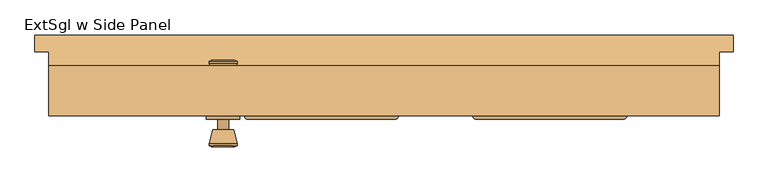
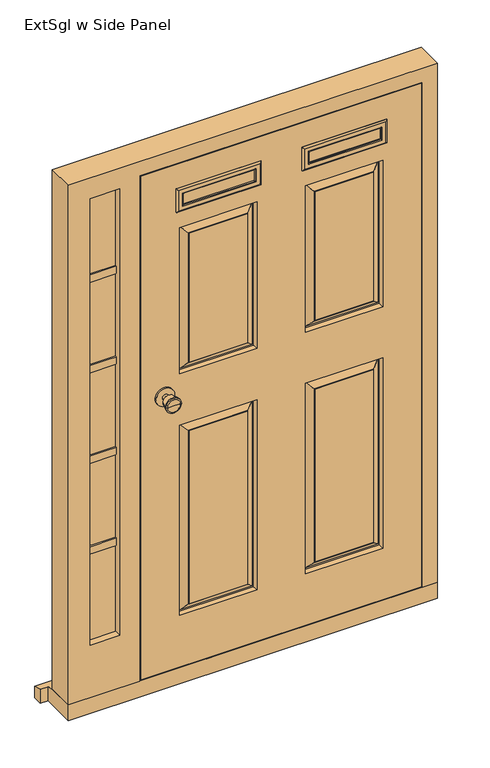
"""IFC4 building model written with IfcOpenShell, lengths in millimetres: door geometry, ExtSgl w Side Panel."""

from ifc_helpers import new_model, si_unit, point, frame, frame_2d, origin, place, context, project, spatial, polyline, circle_curve, ellipse_curve, trimmed, segment, composite_curve, outline, extrude, faceted_brep, source, transform, mapped, element, save
from ifc_brep_helpers import plane_surface, cylinder_surface, revolved_surface, advanced_brep


def extsgl_w_side_panel_d749231e(model_context):
    return source(origin(), model_context, "Body", "SolidModel", [
        advanced_brep(
        [(-518.7, -5.7, 1000.0), (-508.7, -5.7, 1000.0), (-528.7, -5.7, 1000.0), (-498.2241324, -54.7, 1000.0), (-518.7, -54.7, 1000.0), (-539.1758676, -54.7, 1000.0), (-493.7, -52.8721319, 1000.0), (-543.7, -52.8721319, 1000.0), (-493.7, -49.4084537, 1000.0), (-543.7, -49.4084537, 1000.0), (-500.063764, -24.7, 1000.0), (-537.336236, -24.7, 1000.0), (-508.7, -24.7, 1000.0), (-528.7, -24.7, 1000.0)],
        [
            (0, 1),
            (1, 2, circle_curve(frame((-518.7, -5.7, 1000.0), z_axis=(0.0, 1.0, 0.0), x_axis=(-1.0, 0.0, 0.0)), 10.0)),
            (2, 0),
            (2, 1, circle_curve(frame((-518.7, -5.7, 1000.0), z_axis=(0.0, 1.0, 0.0), x_axis=(-1.0, 0.0, 0.0)), 10.0)),
            (3, 4),
            (4, 5),
            (5, 3, circle_curve(frame((-518.7, -54.7, 1000.0), z_axis=(0.0, -1.0, 0.0), x_axis=(-1.0, 0.0, 0.0)), 20.4758676)),
            (3, 5, circle_curve(frame((-518.7, -54.7, 1000.0), z_axis=(0.0, -1.0, 0.0), x_axis=(-1.0, 0.0, 0.0)), 20.4758676)),
            (6, 3),
            (5, 7),
            (7, 6, circle_curve(frame((-518.7, -52.8721319, 1000.0), z_axis=(0.0, -1.0, 0.0), x_axis=(-1.0, 0.0, 0.0)), 25.0)),
            (6, 7, circle_curve(frame((-518.7, -52.8721319, 1000.0), z_axis=(0.0, -1.0, 0.0), x_axis=(-1.0, 0.0, 0.0)), 25.0)),
            (8, 6),
            (7, 9),
            (9, 8, circle_curve(frame((-518.7, -49.4084537, 1000.0), z_axis=(0.0, -1.0, 0.0), x_axis=(-1.0, 0.0, 0.0)), 25.0)),
            (8, 9, circle_curve(frame((-518.7, -49.4084537, 1000.0), z_axis=(0.0, -1.0, 0.0), x_axis=(-1.0, 0.0, 0.0)), 25.0)),
            (10, 8),
            (9, 11),
            (11, 10, circle_curve(frame((-518.7, -24.7, 1000.0), z_axis=(0.0, -1.0, 0.0), x_axis=(-1.0, 0.0, 0.0)), 18.636236)),
            (10, 11, circle_curve(frame((-518.7, -24.7, 1000.0), z_axis=(0.0, -1.0, 0.0), x_axis=(-1.0, 0.0, 0.0)), 18.636236)),
            (12, 10),
            (11, 13),
            (13, 12, circle_curve(frame((-518.7, -24.7, 1000.0), z_axis=(0.0, -1.0, 0.0), x_axis=(-1.0, 0.0, 0.0)), 10.0)),
            (12, 13, circle_curve(frame((-518.7, -24.7, 1000.0), z_axis=(0.0, -1.0, 0.0), x_axis=(-1.0, 0.0, 0.0)), 10.0)),
            (1, 12),
            (13, 2),
        ],
        [
            plane_surface(frame((-518.7, -5.7, 1000.0), z_axis=(0.0, 1.0, 0.0), x_axis=(-1.0, 0.0, 0.0))),
            plane_surface(frame((-518.7, -54.7, 1000.0), z_axis=(0.0, -1.0, 0.0), x_axis=(-1.0, 0.0, 0.0))),
            revolved_surface(polyline([(-539.1758676, -54.7, 1000.0), (-543.7, -52.8721319, 1000.0)]), (-518.7, -5.7, 1000.0), (0.0, 1.0, 0.0)),
            cylinder_surface(frame((-518.7, -5.7, 1000.0), z_axis=(0.0, 1.0, 0.0), x_axis=(-1.0, 0.0, 0.0)), 25.0),
            revolved_surface(polyline([(-543.7, -49.4084537, 1000.0), (-537.336236, -24.7, 1000.0)]), (-518.7, -5.7, 1000.0), (0.0, 1.0, 0.0)),
            plane_surface(frame((-518.7, -24.7, 1000.0), z_axis=(0.0, 1.0, 0.0), x_axis=(-1.0, 0.0, 0.0))),
            cylinder_surface(frame((-518.7, -5.7, 1000.0), z_axis=(0.0, 1.0, 0.0), x_axis=(-1.0, 0.0, 0.0)), 10.0),
        ],
        [
            (0, [[1, 2, 3]]),
            (0, [[-3, 4, -1]]),
            (1, [[5, 6, 7]]),
            (1, [[-6, -5, 8]]),
            (2, [[9, -7, 10, 11]]),
            (2, [[-10, -8, -9, 12]]),
            (3, [[13, -11, 14, 15]]),
            (3, [[-14, -12, -13, 16]]),
            (4, [[17, -15, 18, 19]]),
            (4, [[-18, -16, -17, 20]]),
            (5, [[21, -19, 22, 23]]),
            (5, [[-22, -20, -21, 24]]),
            (6, [[25, -23, 26, -2]]),
            (6, [[-26, -24, -25, -4]]),
        ],
    ),
        extrude(outline(composite_curve([segment(trimmed(circle_curve(frame_2d((1000.0, -518.7)), 30.0), [point((1000.0, -548.7))], [point((1000.0, -488.7))], False, "CARTESIAN"), True, "CONTINUOUS"), segment(trimmed(circle_curve(frame_2d((1000.0, -518.7)), 30.0), [point((1000.0, -488.7))], [point((1000.0, -548.7))], False, "CARTESIAN"), True, "CONTINUOUS")], self_intersect=False)), frame((0.0, -5.7, 0.0), z_axis=(0.0, 1.0, 0.0), x_axis=(0.0, 0.0, 1.0)), (0.0, 0.0, 1.0), 6.0),
        advanced_brep(
        [(-518.7, 50.3, 1000.0), (-528.7, 50.3, 1000.0), (-508.7, 50.3, 1000.0), (-498.2241324, 99.3, 1000.0), (-539.1758676, 99.3, 1000.0), (-518.7, 99.3, 1000.0), (-493.7, 97.4721319, 1000.0), (-543.7, 97.4721319, 1000.0), (-493.7, 94.0084537, 1000.0), (-543.7, 94.0084537, 1000.0), (-500.063764, 69.3, 1000.0), (-537.336236, 69.3, 1000.0), (-508.7, 69.3, 1000.0), (-528.7, 69.3, 1000.0)],
        [
            (0, 1),
            (1, 2, circle_curve(frame((-518.7, 50.3, 1000.0), z_axis=(0.0, -1.0, 0.0), x_axis=(-1.0, 0.0, 0.0)), 10.0)),
            (2, 0),
            (2, 1, circle_curve(frame((-518.7, 50.3, 1000.0), z_axis=(0.0, -1.0, 0.0), x_axis=(-1.0, 0.0, 0.0)), 10.0)),
            (3, 4, circle_curve(frame((-518.7, 99.3, 1000.0), z_axis=(0.0, 1.0, 0.0), x_axis=(-1.0, 0.0, 0.0)), 20.4758676)),
            (4, 5),
            (5, 3),
            (4, 3, circle_curve(frame((-518.7, 99.3, 1000.0), z_axis=(0.0, 1.0, 0.0), x_axis=(-1.0, 0.0, 0.0)), 20.4758676)),
            (6, 7, circle_curve(frame((-518.7, 97.4721319, 1000.0), z_axis=(0.0, 1.0, 0.0), x_axis=(-1.0, 0.0, 0.0)), 25.0)),
            (7, 4),
            (3, 6),
            (7, 6, circle_curve(frame((-518.7, 97.4721319, 1000.0), z_axis=(0.0, 1.0, 0.0), x_axis=(-1.0, 0.0, 0.0)), 25.0)),
            (8, 9, circle_curve(frame((-518.7, 94.0084537, 1000.0), z_axis=(0.0, 1.0, 0.0), x_axis=(-1.0, 0.0, 0.0)), 25.0)),
            (9, 7),
            (6, 8),
            (9, 8, circle_curve(frame((-518.7, 94.0084537, 1000.0), z_axis=(0.0, 1.0, 0.0), x_axis=(-1.0, 0.0, 0.0)), 25.0)),
            (10, 11, circle_curve(frame((-518.7, 69.3, 1000.0), z_axis=(0.0, 1.0, 0.0), x_axis=(-1.0, 0.0, 0.0)), 18.636236)),
            (11, 9),
            (8, 10),
            (11, 10, circle_curve(frame((-518.7, 69.3, 1000.0), z_axis=(0.0, 1.0, 0.0), x_axis=(-1.0, 0.0, 0.0)), 18.636236)),
            (12, 13, circle_curve(frame((-518.7, 69.3, 1000.0), z_axis=(0.0, 1.0, 0.0), x_axis=(-1.0, 0.0, 0.0)), 10.0)),
            (13, 11),
            (10, 12),
            (13, 12, circle_curve(frame((-518.7, 69.3, 1000.0), z_axis=(0.0, 1.0, 0.0), x_axis=(-1.0, 0.0, 0.0)), 10.0)),
            (1, 13),
            (12, 2),
        ],
        [
            plane_surface(frame((-518.7, 50.3, 1000.0), z_axis=(0.0, -1.0, 0.0), x_axis=(-1.0, 0.0, 0.0))),
            plane_surface(frame((-518.7, 99.3, 1000.0), z_axis=(0.0, 1.0, 0.0), x_axis=(-1.0, 0.0, 0.0))),
            revolved_surface(polyline([(-539.1758676, 99.3, 1000.0), (-543.7, 97.4721319, 1000.0)]), (-518.7, 50.3, 1000.0), (0.0, -1.0, 0.0)),
            cylinder_surface(frame((-518.7, 50.3, 1000.0), z_axis=(0.0, -1.0, 0.0), x_axis=(-1.0, 0.0, 0.0)), 25.0),
            revolved_surface(polyline([(-543.7, 94.0084537, 1000.0), (-537.336236, 69.3, 1000.0)]), (-518.7, 50.3, 1000.0), (0.0, -1.0, 0.0)),
            plane_surface(frame((-518.7, 69.3, 1000.0), z_axis=(0.0, -1.0, 0.0), x_axis=(-1.0, 0.0, 0.0))),
            cylinder_surface(frame((-518.7, 50.3, 1000.0), z_axis=(0.0, -1.0, 0.0), x_axis=(-1.0, 0.0, 0.0)), 10.0),
        ],
        [
            (0, [[1, 2, 3]]),
            (0, [[-3, 4, -1]]),
            (1, [[5, 6, 7]]),
            (1, [[8, -7, -6]]),
            (2, [[9, 10, -5, 11]]),
            (2, [[12, -11, -8, -10]]),
            (3, [[13, 14, -9, 15]]),
            (3, [[16, -15, -12, -14]]),
            (4, [[17, 18, -13, 19]]),
            (4, [[20, -19, -16, -18]]),
            (5, [[21, 22, -17, 23]]),
            (5, [[24, -23, -20, -22]]),
            (6, [[-2, 25, -21, 26]]),
            (6, [[-4, -26, -24, -25]]),
        ],
    ),
        extrude(outline(composite_curve([segment(trimmed(circle_curve(frame_2d((1000.0, -518.7)), 30.0), [point((1000.0, -548.7))], [point((1000.0, -488.7))], False, "CARTESIAN"), True, "CONTINUOUS"), segment(trimmed(circle_curve(frame_2d((1000.0, -518.7)), 30.0), [point((1000.0, -488.7))], [point((1000.0, -548.7))], False, "CARTESIAN"), True, "CONTINUOUS")], self_intersect=False)), frame((0.0, 44.3, 0.0), z_axis=(0.0, 1.0, 0.0), x_axis=(0.0, 0.0, 1.0)), (0.0, 0.0, 1.0), 6.0),
        faceted_brep([(294.3, 89.3, 54.5), (364.8, 89.3, 54.5), (364.8, 0.3, 54.5), (316.3, 0.3, 54.5), (316.3, 47.3, 54.5), (294.3, 47.3, 54.5), (294.3, 89.3, 1758.3), (-576.7, 89.3, 1758.3), (-576.7, 89.3, 54.5), (-829.0, 89.3, 54.5), (-829.0, 89.3, 1828.8), (364.8, 89.3, 1828.8), (-662.7, 89.3, 1758.3), (-758.5, 89.3, 1758.3), (-758.5, 89.3, 233.5), (-662.7, 89.3, 233.5), (364.8, 0.3, 1828.8), (-829.0, 0.3, 1828.8), (-829.0, 0.3, 54.5), (-598.7, 0.3, 54.5), (-598.7, 0.3, 1780.3), (316.3, 0.3, 1780.3), (-662.7, 0.3, 233.5), (-758.5, 0.3, 233.5), (-758.5, 0.3, 1758.3), (-662.7, 0.3, 1758.3), (316.3, 47.3, 1780.3), (-598.7, 47.3, 1780.3), (-598.7, 47.3, 54.5), (-576.7, 47.3, 54.5), (-576.7, 47.3, 1758.3), (294.3, 47.3, 1758.3), (-640.7, 47.3, 1780.3), (-780.5, 47.3, 1780.3), (-780.5, 47.3, 218.5), (-640.7, 47.3, 218.5), (-758.5, 47.3, 1758.3), (-662.7, 47.3, 1758.3), (-662.7, 47.3, 233.5), (-758.5, 47.3, 233.5), (-662.7, 23.3, 233.5), (-758.5, 23.3, 233.5), (-758.5, 23.3, 1758.3), (-662.7, 23.3, 1758.3), (-780.5, 23.3, 1780.3), (-780.5, 23.3, 218.5), (-640.7, 23.3, 218.5), (-640.7, 23.3, 1780.3)], [[[0, 1, 2, 3, 4, 5]], [[1, 0, 6, 7, 8, 9, 10, 11], [12, 13, 14, 15]], [[2, 1, 11, 16]], [[3, 2, 16, 17, 18, 19, 20, 21], [22, 23, 24, 25]], [[4, 3, 21, 26]], [[5, 4, 26, 27, 28, 29, 30, 31]], [[32, 33, 34, 35], [36, 37, 38, 39]], [[0, 5, 31, 6]], [[29, 8, 7, 30]], [[18, 9, 8, 29, 28, 19]], [[10, 9, 18, 17]], [[13, 36, 39, 14]], [[39, 38, 15, 14]], [[37, 12, 15, 38]], [[23, 22, 40, 41]], [[24, 23, 41, 42]], [[22, 25, 43, 40]], [[19, 28, 27, 20]], [[44, 45, 34, 33]], [[45, 46, 35, 34]], [[46, 47, 32, 35]], [[46, 45, 44, 47], [41, 40, 43, 42]], [[11, 10, 17, 16]], [[26, 21, 20, 27]], [[33, 32, 47, 44]], [[6, 31, 30, 7]], [[36, 13, 12, 37]], [[25, 24, 42, 43]]]),
        faceted_brep([(313.3, 0.3, 58.5), (313.3, 0.3, 1777.3), (-593.7, 0.3, 1777.3), (-593.7, 0.3, 58.5), (-61.7, 0.3, 1683.5), (188.3, 0.3, 1683.5), (188.3, 0.3, 1627.3), (-61.7, 0.3, 1627.3), (-468.7, 0.3, 1683.5), (-218.7, 0.3, 1683.5), (-218.7, 0.3, 1627.3), (-468.7, 0.3, 1627.3), (-218.7, 0.3, 883.5), (-218.7, 0.3, 233.5), (-468.7, 0.3, 233.5), (-468.7, 0.3, 883.5), (188.3, 0.3, 883.5), (188.3, 0.3, 233.5), (-61.7, 0.3, 233.5), (-61.7, 0.3, 883.5), (-218.7, 0.3, 1558.5), (-218.7, 0.3, 1058.5), (-468.7, 0.3, 1058.5), (-468.7, 0.3, 1558.5), (188.3, 0.3, 1558.5), (188.3, 0.3, 1058.5), (-61.7, 0.3, 1058.5), (-61.7, 0.3, 1558.5), (-248.7, 0.3, 263.5), (-248.7, 0.3, 853.5), (-438.7, 0.3, 853.5), (-438.7, 0.3, 263.5), (158.3, 0.3, 263.5), (158.3, 0.3, 853.5), (-31.7, 0.3, 853.5), (-31.7, 0.3, 263.5), (-248.7, 0.3, 1088.5), (-248.7, 0.3, 1528.5), (-438.7, 0.3, 1528.5), (-438.7, 0.3, 1088.5), (158.3, 0.3, 1088.5), (158.3, 0.3, 1528.5), (-31.7, 0.3, 1528.5), (-31.7, 0.3, 1088.5), (313.3, 44.3, 58.5), (-593.7, 44.3, 58.5), (-593.7, 44.3, 1777.3), (313.3, 44.3, 1777.3), (-61.7, 44.3, 1683.5), (-61.7, 44.3, 1627.3), (188.3, 44.3, 1627.3), (188.3, 44.3, 1683.5), (-468.7, 44.3, 1683.5), (-468.7, 44.3, 1627.3), (-218.7, 44.3, 1627.3), (-218.7, 44.3, 1683.5), (-61.7, 44.3, 883.5), (-61.7, 44.3, 233.5), (188.3, 44.3, 233.5), (188.3, 44.3, 883.5), (-468.7, 44.3, 883.5), (-468.7, 44.3, 233.5), (-218.7, 44.3, 233.5), (-218.7, 44.3, 883.5), (-61.7, 44.3, 1558.5), (-61.7, 44.3, 1058.5), (188.3, 44.3, 1058.5), (188.3, 44.3, 1558.5), (-468.7, 44.3, 1558.5), (-468.7, 44.3, 1058.5), (-218.7, 44.3, 1058.5), (-218.7, 44.3, 1558.5), (-31.7, 44.3, 263.5), (-31.7, 44.3, 853.5), (158.3, 44.3, 853.5), (158.3, 44.3, 263.5), (-438.7, 44.3, 263.5), (-438.7, 44.3, 853.5), (-248.7, 44.3, 853.5), (-248.7, 44.3, 263.5), (-31.7, 44.3, 1088.5), (-31.7, 44.3, 1528.5), (158.3, 44.3, 1528.5), (158.3, 44.3, 1088.5), (-438.7, 44.3, 1088.5), (-438.7, 44.3, 1528.5), (-248.7, 44.3, 1528.5), (-248.7, 44.3, 1088.5), (-58.7, 29.3, 880.5), (-58.7, 29.3, 236.5), (-33.7, 43.3, 855.5), (-33.7, 43.3, 261.5), (-53.7, 29.3, 241.5), (-53.7, 29.3, 875.5), (-31.7, 43.3, 263.5), (-31.7, 43.3, 853.5), (185.3, 29.3, 236.5), (160.3, 43.3, 261.5), (180.3, 29.3, 241.5), (158.3, 43.3, 263.5), (185.3, 29.3, 880.5), (160.3, 43.3, 855.5), (180.3, 29.3, 875.5), (158.3, 43.3, 853.5), (-465.7, 29.3, 880.5), (-465.7, 29.3, 236.5), (-440.7, 43.3, 855.5), (-440.7, 43.3, 261.5), (-460.7, 29.3, 241.5), (-460.7, 29.3, 875.5), (-438.7, 43.3, 263.5), (-438.7, 43.3, 853.5), (-221.7, 29.3, 236.5), (-246.7, 43.3, 261.5), (-226.7, 29.3, 241.5), (-248.7, 43.3, 263.5), (-221.7, 29.3, 880.5), (-246.7, 43.3, 855.5), (-226.7, 29.3, 875.5), (-248.7, 43.3, 853.5), (-248.7, 1.3, 263.5), (-248.7, 1.3, 853.5), (-226.7, 15.3, 241.5), (-226.7, 15.3, 875.5), (-246.7, 1.3, 855.5), (-246.7, 1.3, 261.5), (-221.7, 15.3, 880.5), (-221.7, 15.3, 236.5), (-438.7, 1.3, 853.5), (-460.7, 15.3, 875.5), (-440.7, 1.3, 855.5), (-465.7, 15.3, 880.5), (-438.7, 1.3, 263.5), (-460.7, 15.3, 241.5), (-440.7, 1.3, 261.5), (-465.7, 15.3, 236.5), (185.3, 15.3, 880.5), (185.3, 15.3, 236.5), (160.3, 1.3, 855.5), (160.3, 1.3, 261.5), (180.3, 15.3, 241.5), (180.3, 15.3, 875.5), (158.3, 1.3, 263.5), (158.3, 1.3, 853.5), (-58.7, 15.3, 236.5), (-33.7, 1.3, 261.5), (-53.7, 15.3, 241.5), (-31.7, 1.3, 263.5), (-58.7, 15.3, 880.5), (-33.7, 1.3, 855.5), (-53.7, 15.3, 875.5), (-31.7, 1.3, 853.5), (-31.7, 43.3, 1088.5), (-31.7, 43.3, 1528.5), (-53.7, 29.3, 1066.5), (-53.7, 29.3, 1550.5), (-33.7, 43.3, 1530.5), (-33.7, 43.3, 1086.5), (-58.7, 29.3, 1555.5), (-58.7, 29.3, 1061.5), (158.3, 43.3, 1528.5), (180.3, 29.3, 1550.5), (160.3, 43.3, 1530.5), (185.3, 29.3, 1555.5), (158.3, 43.3, 1088.5), (180.3, 29.3, 1066.5), (160.3, 43.3, 1086.5), (185.3, 29.3, 1061.5), (-438.7, 43.3, 1088.5), (-438.7, 43.3, 1528.5), (-460.7, 29.3, 1066.5), (-460.7, 29.3, 1550.5), (-440.7, 43.3, 1530.5), (-440.7, 43.3, 1086.5), (-465.7, 29.3, 1555.5), (-465.7, 29.3, 1061.5), (-248.7, 43.3, 1528.5), (-226.7, 29.3, 1550.5), (-246.7, 43.3, 1530.5), (-221.7, 29.3, 1555.5), (-248.7, 43.3, 1088.5), (-226.7, 29.3, 1066.5), (-246.7, 43.3, 1086.5), (-221.7, 29.3, 1061.5), (-248.7, 1.3, 1088.5), (-248.7, 1.3, 1528.5), (-226.7, 15.3, 1066.5), (-226.7, 15.3, 1550.5), (-246.7, 1.3, 1530.5), (-246.7, 1.3, 1086.5), (-221.7, 15.3, 1555.5), (-221.7, 15.3, 1061.5), (-438.7, 1.3, 1528.5), (-460.7, 15.3, 1550.5), (-440.7, 1.3, 1530.5), (-465.7, 15.3, 1555.5), (-438.7, 1.3, 1088.5), (-460.7, 15.3, 1066.5), (-440.7, 1.3, 1086.5), (-465.7, 15.3, 1061.5), (185.3, 15.3, 1555.5), (185.3, 15.3, 1061.5), (160.3, 1.3, 1530.5), (160.3, 1.3, 1086.5), (180.3, 15.3, 1066.5), (180.3, 15.3, 1550.5), (158.3, 1.3, 1088.5), (158.3, 1.3, 1528.5), (-58.7, 15.3, 1061.5), (-33.7, 1.3, 1086.5), (-53.7, 15.3, 1066.5), (-31.7, 1.3, 1088.5), (-58.7, 15.3, 1555.5), (-33.7, 1.3, 1530.5), (-53.7, 15.3, 1550.5), (-31.7, 1.3, 1528.5)], [[[0, 1, 2, 3], [4, 5, 6, 7], [8, 9, 10, 11], [12, 13, 14, 15], [16, 17, 18, 19], [20, 21, 22, 23], [24, 25, 26, 27]], [[28, 29, 30, 31]], [[32, 33, 34, 35]], [[36, 37, 38, 39]], [[40, 41, 42, 43]], [[44, 45, 46, 47], [48, 49, 50, 51], [52, 53, 54, 55], [56, 57, 58, 59], [60, 61, 62, 63], [64, 65, 66, 67], [68, 69, 70, 71]], [[72, 73, 74, 75]], [[76, 77, 78, 79]], [[80, 81, 82, 83]], [[84, 85, 86, 87]], [[1, 0, 44, 47]], [[2, 1, 47, 46]], [[3, 2, 46, 45]], [[0, 3, 45, 44]], [[4, 7, 49, 48]], [[7, 6, 50, 49]], [[6, 5, 51, 50]], [[5, 4, 48, 51]], [[8, 11, 53, 52]], [[11, 10, 54, 53]], [[10, 9, 55, 54]], [[9, 8, 52, 55]], [[88, 89, 57, 56]], [[90, 91, 92, 93]], [[72, 94, 95, 73]], [[57, 89, 96, 58]], [[92, 91, 97, 98]], [[94, 72, 75, 99]], [[58, 96, 100, 59]], [[98, 97, 101, 102]], [[99, 75, 74, 103]], [[88, 56, 59, 100]], [[89, 88, 100, 96], [93, 92, 98, 102]], [[90, 93, 102, 101]], [[91, 90, 101, 97], [95, 94, 99, 103]], [[73, 95, 103, 74]], [[104, 105, 61, 60]], [[106, 107, 108, 109]], [[76, 110, 111, 77]], [[61, 105, 112, 62]], [[108, 107, 113, 114]], [[110, 76, 79, 115]], [[62, 112, 116, 63]], [[114, 113, 117, 118]], [[115, 79, 78, 119]], [[104, 60, 63, 116]], [[105, 104, 116, 112], [109, 108, 114, 118]], [[106, 109, 118, 117]], [[107, 106, 117, 113], [111, 110, 115, 119]], [[77, 111, 119, 78]], [[120, 121, 29, 28]], [[122, 123, 124, 125]], [[12, 126, 127, 13]], [[29, 121, 128, 30]], [[124, 123, 129, 130]], [[126, 12, 15, 131]], [[30, 128, 132, 31]], [[130, 129, 133, 134]], [[131, 15, 14, 135]], [[120, 28, 31, 132]], [[125, 124, 130, 134], [121, 120, 132, 128]], [[122, 125, 134, 133]], [[127, 126, 131, 135], [123, 122, 133, 129]], [[13, 127, 135, 14]], [[136, 137, 17, 16]], [[138, 139, 140, 141]], [[32, 142, 143, 33]], [[17, 137, 144, 18]], [[140, 139, 145, 146]], [[142, 32, 35, 147]], [[18, 144, 148, 19]], [[146, 145, 149, 150]], [[147, 35, 34, 151]], [[136, 16, 19, 148]], [[137, 136, 148, 144], [141, 140, 146, 150]], [[138, 141, 150, 149]], [[139, 138, 149, 145], [143, 142, 147, 151]], [[33, 143, 151, 34]], [[152, 153, 81, 80]], [[154, 155, 156, 157]], [[64, 158, 159, 65]], [[81, 153, 160, 82]], [[156, 155, 161, 162]], [[158, 64, 67, 163]], [[82, 160, 164, 83]], [[162, 161, 165, 166]], [[163, 67, 66, 167]], [[152, 80, 83, 164]], [[157, 156, 162, 166], [153, 152, 164, 160]], [[154, 157, 166, 165]], [[159, 158, 163, 167], [155, 154, 165, 161]], [[65, 159, 167, 66]], [[168, 169, 85, 84]], [[170, 171, 172, 173]], [[68, 174, 175, 69]], [[85, 169, 176, 86]], [[172, 171, 177, 178]], [[174, 68, 71, 179]], [[86, 176, 180, 87]], [[178, 177, 181, 182]], [[179, 71, 70, 183]], [[168, 84, 87, 180]], [[173, 172, 178, 182], [169, 168, 180, 176]], [[170, 173, 182, 181]], [[175, 174, 179, 183], [171, 170, 181, 177]], [[69, 175, 183, 70]], [[184, 185, 37, 36]], [[186, 187, 188, 189]], [[20, 190, 191, 21]], [[37, 185, 192, 38]], [[188, 187, 193, 194]], [[190, 20, 23, 195]], [[38, 192, 196, 39]], [[194, 193, 197, 198]], [[195, 23, 22, 199]], [[184, 36, 39, 196]], [[189, 188, 194, 198], [185, 184, 196, 192]], [[186, 189, 198, 197]], [[191, 190, 195, 199], [187, 186, 197, 193]], [[21, 191, 199, 22]], [[200, 201, 25, 24]], [[202, 203, 204, 205]], [[40, 206, 207, 41]], [[25, 201, 208, 26]], [[204, 203, 209, 210]], [[206, 40, 43, 211]], [[26, 208, 212, 27]], [[210, 209, 213, 214]], [[211, 43, 42, 215]], [[200, 24, 27, 212]], [[201, 200, 212, 208], [205, 204, 210, 214]], [[202, 205, 214, 213]], [[203, 202, 213, 209], [207, 206, 211, 215]], [[41, 207, 215, 42]]]),
        faceted_brep([(389.8, 144.3, 0.0), (389.8, 144.3, 38.5947221), (389.8, 114.3, 47.2703282), (389.8, 114.3, 0.0), (-854.0, 144.3, 38.5947221), (-854.0, 144.3, 0.0), (-854.0, 114.3, 0.0), (-854.0, 114.3, 47.2703282), (364.8, 114.3, 0.0), (364.8, 0.3, 0.0), (-829.0, 0.3, 0.0), (-829.0, 114.3, 0.0), (-829.0, 114.3, 47.2703282), (-829.0, 89.3, 54.5), (364.8, 89.3, 54.5), (364.8, 114.3, 47.2703282), (-829.0, 0.3, 54.5), (364.8, 0.3, 54.5)], [[[0, 1, 2, 3]], [[4, 5, 6, 7]], [[5, 0, 3, 8, 9, 10, 11, 6]], [[1, 0, 5, 4]], [[1, 4, 7, 12, 13, 14, 15, 2]], [[13, 16, 17, 14]], [[16, 10, 9, 17]], [[12, 11, 10, 16, 13]], [[11, 12, 7, 6]], [[8, 15, 14, 17, 9]], [[15, 8, 3, 2]]]),
        extrude(outline(polyline([(188.3, 10.3), (-61.7, 10.3), (-61.7, 34.3), (188.3, 34.3), (188.3, 10.3)])), frame((0.0, 0.0, 1627.3), z_axis=(0.0, 0.0, 1.0), x_axis=(1.0, 0.0, 0.0)), (0.0, 0.0, 1.0), 56.2),
        extrude(outline(polyline([(-218.7, 10.3), (-468.7, 10.3), (-468.7, 34.3), (-218.7, 34.3), (-218.7, 10.3)])), frame((0.0, 0.0, 1627.3), z_axis=(0.0, 0.0, 1.0), x_axis=(1.0, 0.0, 0.0)), (0.0, 0.0, 1.0), 56.2),
        advanced_brep(
        [(-53.7, 48.3, 1675.5), (-53.7, 44.3, 1675.5), (-53.7, 44.3, 1635.3), (-53.7, 48.3, 1635.3), (-55.7, 50.3, 1677.5), (-55.7, 50.3, 1633.3), (-73.7, 45.3, 1695.5), (-68.7, 50.3, 1690.5), (-68.7, 50.3, 1620.3), (-73.7, 45.3, 1615.3), (-73.7, 34.3, 1695.5), (-73.7, 34.3, 1615.3), (-61.7, 44.3, 1683.5), (-61.7, 34.3, 1683.5), (-61.7, 34.3, 1627.3), (-61.7, 44.3, 1627.3), (180.3, 44.3, 1635.3), (180.3, 48.3, 1635.3), (182.3, 50.3, 1633.3), (195.3, 50.3, 1620.3), (200.3, 45.3, 1615.3), (200.3, 34.3, 1615.3), (188.3, 34.3, 1627.3), (188.3, 44.3, 1627.3), (180.3, 44.3, 1675.5), (180.3, 48.3, 1675.5), (182.3, 50.3, 1677.5), (195.3, 50.3, 1690.5), (200.3, 45.3, 1695.5), (200.3, 34.3, 1695.5), (188.3, 34.3, 1683.5), (188.3, 44.3, 1683.5)],
        [
            (0, 1),
            (1, 2),
            (2, 3),
            (3, 0),
            (4, 0, ellipse_curve(frame((-55.7, 48.3, 1677.5), z_axis=(-0.7071067811865475, 0.0, -0.7071067811865475), x_axis=(-0.7071067811865474, 0.0, 0.7071067811865476)), 2.8284271, 2.0)),
            (3, 5, ellipse_curve(frame((-55.7, 48.3, 1633.3), z_axis=(-0.7071067811865475, 0.0, 0.7071067811865475), x_axis=(0.7071067811865474, 0.0, 0.7071067811865476)), 2.8284271, 2.0)),
            (5, 4),
            (6, 7, ellipse_curve(frame((-68.7, 45.3, 1690.5), z_axis=(-0.7071067811865475, 0.0, -0.7071067811865475), x_axis=(-0.7071067811865474, 0.0, 0.7071067811865476)), 7.0710678, 5.0)),
            (7, 8),
            (8, 9, ellipse_curve(frame((-68.7, 45.3, 1620.3), z_axis=(-0.7071067811865475, 0.0, 0.7071067811865475), x_axis=(0.7071067811865474, 0.0, 0.7071067811865476)), 7.0710678, 5.0)),
            (9, 6),
            (10, 6),
            (9, 11),
            (11, 10),
            (12, 13),
            (13, 14),
            (14, 15),
            (15, 12),
            (2, 16),
            (16, 17),
            (17, 3),
            (17, 18, ellipse_curve(frame((182.3, 48.3, 1633.3), z_axis=(-0.7071067811865475, 0.0, -0.7071067811865475), x_axis=(-0.7071067811865476, 0.0, 0.7071067811865474)), 2.8284271, 2.0)),
            (18, 5),
            (8, 19),
            (19, 20, ellipse_curve(frame((195.3, 45.3, 1620.3), z_axis=(-0.7071067811865475, 0.0, -0.7071067811865475), x_axis=(-0.7071067811865476, 0.0, 0.7071067811865474)), 7.0710678, 5.0)),
            (20, 9),
            (20, 21),
            (21, 11),
            (14, 22),
            (22, 23),
            (23, 15),
            (16, 24),
            (24, 25),
            (25, 17),
            (25, 26, ellipse_curve(frame((182.3, 48.3, 1677.5), z_axis=(0.7071067811865475, 0.0, -0.7071067811865475), x_axis=(-0.7071067811865474, 0.0, -0.7071067811865476)), 2.8284271, 2.0)),
            (26, 18),
            (19, 27),
            (27, 28, ellipse_curve(frame((195.3, 45.3, 1690.5), z_axis=(0.7071067811865475, 0.0, -0.7071067811865475), x_axis=(-0.7071067811865474, 0.0, -0.7071067811865476)), 7.0710678, 5.0)),
            (28, 20),
            (28, 29),
            (29, 21),
            (22, 30),
            (30, 31),
            (31, 23),
            (24, 1),
            (0, 25),
            (4, 26),
            (7, 27),
            (6, 28),
            (10, 29),
            (13, 30),
            (12, 31),
        ],
        [
            plane_surface(frame((-53.7, 44.3, 1675.5), z_axis=(1.0, 0.0, 0.0), x_axis=(0.0, 0.0, -1.0))),
            cylinder_surface(frame((-55.7, 48.3, 1683.5), z_axis=(0.0, 0.0, 1.0), x_axis=(1.0, 0.0, 0.0)), 2.0),
            cylinder_surface(frame((-68.7, 45.3, 1683.5), z_axis=(0.0, 0.0, 1.0), x_axis=(1.0, 0.0, 0.0)), 5.0),
            plane_surface(frame((-73.7, 45.3, 1695.5), z_axis=(-1.0, 0.0, 0.0), x_axis=(0.0, 0.0, -1.0))),
            plane_surface(frame((-61.7, 34.3, 1683.5), z_axis=(1.0, 0.0, 0.0), x_axis=(0.0, 0.0, -1.0))),
            plane_surface(frame((-53.7, 44.3, 1635.3), z_axis=(0.0, 0.0, 1.0), x_axis=(1.0, 0.0, 0.0))),
            cylinder_surface(frame((-61.7, 48.3, 1633.3), z_axis=(-1.0, 0.0, 0.0), x_axis=(0.0, 0.0, 1.0)), 2.0),
            cylinder_surface(frame((-61.7, 45.3, 1620.3), z_axis=(-1.0, 0.0, 0.0), x_axis=(0.0, 0.0, 1.0)), 5.0),
            plane_surface(frame((-73.7, 45.3, 1615.3), z_axis=(0.0, 0.0, -1.0), x_axis=(1.0, 0.0, 0.0))),
            plane_surface(frame((-61.7, 34.3, 1627.3), z_axis=(0.0, 0.0, 1.0), x_axis=(1.0, 0.0, 0.0))),
            plane_surface(frame((180.3, 44.3, 1635.3), z_axis=(-1.0, 0.0, 0.0), x_axis=(0.0, 0.0, 1.0))),
            cylinder_surface(frame((182.3, 48.3, 1627.3), z_axis=(0.0, 0.0, -1.0), x_axis=(-1.0, 0.0, 0.0)), 2.0),
            cylinder_surface(frame((195.3, 45.3, 1627.3), z_axis=(0.0, 0.0, -1.0), x_axis=(-1.0, 0.0, 0.0)), 5.0),
            plane_surface(frame((200.3, 45.3, 1615.3), z_axis=(1.0, 0.0, 0.0), x_axis=(0.0, 0.0, 1.0))),
            plane_surface(frame((188.3, 34.3, 1627.3), z_axis=(-1.0, 0.0, 0.0), x_axis=(0.0, 0.0, 1.0))),
            plane_surface(frame((180.3, 44.3, 1675.5), z_axis=(0.0, 0.0, -1.0), x_axis=(-1.0, 0.0, 0.0))),
            cylinder_surface(frame((188.3, 48.3, 1677.5), z_axis=(1.0, 0.0, 0.0), x_axis=(0.0, 0.0, -1.0)), 2.0),
            plane_surface(frame((182.3, 50.3, 1677.5), z_axis=(0.0, 1.0, 0.0), x_axis=(-1.0, 0.0, 0.0))),
            cylinder_surface(frame((188.3, 45.3, 1690.5), z_axis=(1.0, 0.0, 0.0), x_axis=(0.0, 0.0, -1.0)), 5.0),
            plane_surface(frame((200.3, 45.3, 1695.5), z_axis=(0.0, 0.0, 1.0), x_axis=(-1.0, 0.0, 0.0))),
            plane_surface(frame((200.3, 34.3, 1695.5), z_axis=(0.0, -1.0, 0.0), x_axis=(-1.0, 0.0, 0.0))),
            plane_surface(frame((188.3, 34.3, 1683.5), z_axis=(0.0, 0.0, -1.0), x_axis=(-1.0, 0.0, 0.0))),
            plane_surface(frame((188.3, 44.3, 1683.5), z_axis=(0.0, -1.0, 0.0), x_axis=(-1.0, 0.0, 0.0))),
        ],
        [
            (0, [[1, 2, 3, 4]]),
            (1, [[5, -4, 6, 7]]),
            (2, [[8, 9, 10, 11]]),
            (3, [[12, -11, 13, 14]]),
            (4, [[15, 16, 17, 18]]),
            (5, [[-3, 19, 20, 21]]),
            (6, [[-6, -21, 22, 23]]),
            (7, [[-10, 24, 25, 26]]),
            (8, [[-13, -26, 27, 28]]),
            (9, [[-17, 29, 30, 31]]),
            (10, [[-20, 32, 33, 34]]),
            (11, [[-22, -34, 35, 36]]),
            (12, [[-25, 37, 38, 39]]),
            (13, [[-27, -39, 40, 41]]),
            (14, [[-30, 42, 43, 44]]),
            (15, [[-33, 45, -1, 46]]),
            (16, [[-35, -46, -5, 47]]),
            (17, [[48, -37, -24, -9], [-23, -36, -47, -7]]),
            (18, [[-38, -48, -8, 49]]),
            (19, [[-40, -49, -12, 50]]),
            (20, [[-28, -41, -50, -14], [51, -42, -29, -16]]),
            (21, [[-43, -51, -15, 52]]),
            (22, [[-31, -44, -52, -18], [-45, -32, -19, -2]]),
        ],
    ),
        advanced_brep(
        [(-460.7, 48.3, 1675.5), (-460.7, 44.3, 1675.5), (-460.7, 44.3, 1635.3), (-460.7, 48.3, 1635.3), (-462.7, 50.3, 1677.5), (-462.7, 50.3, 1633.3), (-480.7, 45.3, 1695.5), (-475.7, 50.3, 1690.5), (-475.7, 50.3, 1620.3), (-480.7, 45.3, 1615.3), (-480.7, 34.3, 1695.5), (-480.7, 34.3, 1615.3), (-468.7, 44.3, 1683.5), (-468.7, 34.3, 1683.5), (-468.7, 34.3, 1627.3), (-468.7, 44.3, 1627.3), (-226.7, 44.3, 1635.3), (-226.7, 48.3, 1635.3), (-224.7, 50.3, 1633.3), (-211.7, 50.3, 1620.3), (-206.7, 45.3, 1615.3), (-206.7, 34.3, 1615.3), (-218.7, 34.3, 1627.3), (-218.7, 44.3, 1627.3), (-226.7, 44.3, 1675.5), (-226.7, 48.3, 1675.5), (-224.7, 50.3, 1677.5), (-211.7, 50.3, 1690.5), (-206.7, 45.3, 1695.5), (-206.7, 34.3, 1695.5), (-218.7, 34.3, 1683.5), (-218.7, 44.3, 1683.5)],
        [
            (0, 1),
            (1, 2),
            (2, 3),
            (3, 0),
            (4, 0, ellipse_curve(frame((-462.7, 48.3, 1677.5), z_axis=(-0.7071067811865475, 0.0, -0.7071067811865475), x_axis=(-0.7071067811865474, 0.0, 0.7071067811865476)), 2.8284271, 2.0)),
            (3, 5, ellipse_curve(frame((-462.7, 48.3, 1633.3), z_axis=(-0.7071067811865475, 0.0, 0.7071067811865475), x_axis=(0.7071067811865474, 0.0, 0.7071067811865476)), 2.8284271, 2.0)),
            (5, 4),
            (6, 7, ellipse_curve(frame((-475.7, 45.3, 1690.5), z_axis=(-0.7071067811865475, 0.0, -0.7071067811865475), x_axis=(-0.7071067811865474, 0.0, 0.7071067811865476)), 7.0710678, 5.0)),
            (7, 8),
            (8, 9, ellipse_curve(frame((-475.7, 45.3, 1620.3), z_axis=(-0.7071067811865475, 0.0, 0.7071067811865475), x_axis=(0.7071067811865474, 0.0, 0.7071067811865476)), 7.0710678, 5.0)),
            (9, 6),
            (10, 6),
            (9, 11),
            (11, 10),
            (12, 13),
            (13, 14),
            (14, 15),
            (15, 12),
            (2, 16),
            (16, 17),
            (17, 3),
            (17, 18, ellipse_curve(frame((-224.7, 48.3, 1633.3), z_axis=(-0.7071067811865475, 0.0, -0.7071067811865475), x_axis=(-0.7071067811865476, 0.0, 0.7071067811865474)), 2.8284271, 2.0)),
            (18, 5),
            (8, 19),
            (19, 20, ellipse_curve(frame((-211.7, 45.3, 1620.3), z_axis=(-0.7071067811865475, 0.0, -0.7071067811865475), x_axis=(-0.7071067811865476, 0.0, 0.7071067811865474)), 7.0710678, 5.0)),
            (20, 9),
            (20, 21),
            (21, 11),
            (14, 22),
            (22, 23),
            (23, 15),
            (16, 24),
            (24, 25),
            (25, 17),
            (25, 26, ellipse_curve(frame((-224.7, 48.3, 1677.5), z_axis=(0.7071067811865475, 0.0, -0.7071067811865475), x_axis=(-0.7071067811865474, 0.0, -0.7071067811865476)), 2.8284271, 2.0)),
            (26, 18),
            (19, 27),
            (27, 28, ellipse_curve(frame((-211.7, 45.3, 1690.5), z_axis=(0.7071067811865475, 0.0, -0.7071067811865475), x_axis=(-0.7071067811865474, 0.0, -0.7071067811865476)), 7.0710678, 5.0)),
            (28, 20),
            (28, 29),
            (29, 21),
            (22, 30),
            (30, 31),
            (31, 23),
            (24, 1),
            (0, 25),
            (4, 26),
            (7, 27),
            (6, 28),
            (10, 29),
            (13, 30),
            (12, 31),
        ],
        [
            plane_surface(frame((-460.7, 44.3, 1675.5), z_axis=(1.0, 0.0, 0.0), x_axis=(0.0, 0.0, -1.0))),
            cylinder_surface(frame((-462.7, 48.3, 1683.5), z_axis=(0.0, 0.0, 1.0), x_axis=(1.0, 0.0, 0.0)), 2.0),
            cylinder_surface(frame((-475.7, 45.3, 1683.5), z_axis=(0.0, 0.0, 1.0), x_axis=(1.0, 0.0, 0.0)), 5.0),
            plane_surface(frame((-480.7, 45.3, 1695.5), z_axis=(-1.0, 0.0, 0.0), x_axis=(0.0, 0.0, -1.0))),
            plane_surface(frame((-468.7, 34.3, 1683.5), z_axis=(1.0, 0.0, 0.0), x_axis=(0.0, 0.0, -1.0))),
            plane_surface(frame((-460.7, 44.3, 1635.3), z_axis=(0.0, 0.0, 1.0), x_axis=(1.0, 0.0, 0.0))),
            cylinder_surface(frame((-468.7, 48.3, 1633.3), z_axis=(-1.0, 0.0, 0.0), x_axis=(0.0, 0.0, 1.0)), 2.0),
            cylinder_surface(frame((-468.7, 45.3, 1620.3), z_axis=(-1.0, 0.0, 0.0), x_axis=(0.0, 0.0, 1.0)), 5.0),
            plane_surface(frame((-480.7, 45.3, 1615.3), z_axis=(0.0, 0.0, -1.0), x_axis=(1.0, 0.0, 0.0))),
            plane_surface(frame((-468.7, 34.3, 1627.3), z_axis=(0.0, 0.0, 1.0), x_axis=(1.0, 0.0, 0.0))),
            plane_surface(frame((-226.7, 44.3, 1635.3), z_axis=(-1.0, 0.0, 0.0), x_axis=(0.0, 0.0, 1.0))),
            cylinder_surface(frame((-224.7, 48.3, 1627.3), z_axis=(0.0, 0.0, -1.0), x_axis=(-1.0, 0.0, 0.0)), 2.0),
            cylinder_surface(frame((-211.7, 45.3, 1627.3), z_axis=(0.0, 0.0, -1.0), x_axis=(-1.0, 0.0, 0.0)), 5.0),
            plane_surface(frame((-206.7, 45.3, 1615.3), z_axis=(1.0, 0.0, 0.0), x_axis=(0.0, 0.0, 1.0))),
            plane_surface(frame((-218.7, 34.3, 1627.3), z_axis=(-1.0, 0.0, 0.0), x_axis=(0.0, 0.0, 1.0))),
            plane_surface(frame((-226.7, 44.3, 1675.5), z_axis=(0.0, 0.0, -1.0), x_axis=(-1.0, 0.0, 0.0))),
            cylinder_surface(frame((-218.7, 48.3, 1677.5), z_axis=(1.0, 0.0, 0.0), x_axis=(0.0, 0.0, -1.0)), 2.0),
            plane_surface(frame((-224.7, 50.3, 1677.5), z_axis=(0.0, 1.0, 0.0), x_axis=(-1.0, 0.0, 0.0))),
            cylinder_surface(frame((-218.7, 45.3, 1690.5), z_axis=(1.0, 0.0, 0.0), x_axis=(0.0, 0.0, -1.0)), 5.0),
            plane_surface(frame((-206.7, 45.3, 1695.5), z_axis=(0.0, 0.0, 1.0), x_axis=(-1.0, 0.0, 0.0))),
            plane_surface(frame((-206.7, 34.3, 1695.5), z_axis=(0.0, -1.0, 0.0), x_axis=(-1.0, 0.0, 0.0))),
            plane_surface(frame((-218.7, 34.3, 1683.5), z_axis=(0.0, 0.0, -1.0), x_axis=(-1.0, 0.0, 0.0))),
            plane_surface(frame((-218.7, 44.3, 1683.5), z_axis=(0.0, -1.0, 0.0), x_axis=(-1.0, 0.0, 0.0))),
        ],
        [
            (0, [[1, 2, 3, 4]]),
            (1, [[5, -4, 6, 7]]),
            (2, [[8, 9, 10, 11]]),
            (3, [[12, -11, 13, 14]]),
            (4, [[15, 16, 17, 18]]),
            (5, [[-3, 19, 20, 21]]),
            (6, [[-6, -21, 22, 23]]),
            (7, [[-10, 24, 25, 26]]),
            (8, [[-13, -26, 27, 28]]),
            (9, [[-17, 29, 30, 31]]),
            (10, [[-20, 32, 33, 34]]),
            (11, [[-22, -34, 35, 36]]),
            (12, [[-25, 37, 38, 39]]),
            (13, [[-27, -39, 40, 41]]),
            (14, [[-30, 42, 43, 44]]),
            (15, [[-33, 45, -1, 46]]),
            (16, [[-35, -46, -5, 47]]),
            (17, [[48, -37, -24, -9], [-23, -36, -47, -7]]),
            (18, [[-38, -48, -8, 49]]),
            (19, [[-40, -49, -12, 50]]),
            (20, [[-28, -41, -50, -14], [51, -42, -29, -16]]),
            (21, [[-43, -51, -15, 52]]),
            (22, [[-31, -44, -52, -18], [-45, -32, -19, -2]]),
        ],
    ),
        advanced_brep(
        [(-226.7, -3.7, 1675.5), (-226.7, 0.3, 1675.5), (-226.7, 0.3, 1635.3), (-226.7, -3.7, 1635.3), (-224.7, -5.7, 1677.5), (-224.7, -5.7, 1633.3), (-206.7, -0.7, 1695.5), (-211.7, -5.7, 1690.5), (-211.7, -5.7, 1620.3), (-206.7, -0.7, 1615.3), (-206.7, 10.3, 1695.5), (-206.7, 10.3, 1615.3), (-218.7, 0.3, 1683.5), (-218.7, 10.3, 1683.5), (-218.7, 10.3, 1627.3), (-218.7, 0.3, 1627.3), (-460.7, 0.3, 1635.3), (-460.7, -3.7, 1635.3), (-462.7, -5.7, 1633.3), (-475.7, -5.7, 1620.3), (-480.7, -0.7, 1615.3), (-480.7, 10.3, 1615.3), (-468.7, 10.3, 1627.3), (-468.7, 0.3, 1627.3), (-460.7, 0.3, 1675.5), (-460.7, -3.7, 1675.5), (-462.7, -5.7, 1677.5), (-475.7, -5.7, 1690.5), (-480.7, -0.7, 1695.5), (-480.7, 10.3, 1695.5), (-468.7, 10.3, 1683.5), (-468.7, 0.3, 1683.5)],
        [
            (0, 1),
            (1, 2),
            (2, 3),
            (3, 0),
            (4, 0, ellipse_curve(frame((-224.7, -3.7, 1677.5), z_axis=(0.7071067811865475, 0.0, -0.7071067811865475), x_axis=(0.7071067811865474, 0.0, 0.7071067811865476)), 2.8284271, 2.0)),
            (3, 5, ellipse_curve(frame((-224.7, -3.7, 1633.3), z_axis=(0.7071067811865475, 0.0, 0.7071067811865475), x_axis=(-0.7071067811865474, 0.0, 0.7071067811865476)), 2.8284271, 2.0)),
            (5, 4),
            (6, 7, ellipse_curve(frame((-211.7, -0.7, 1690.5), z_axis=(0.7071067811865475, 0.0, -0.7071067811865475), x_axis=(0.7071067811865474, 0.0, 0.7071067811865476)), 7.0710678, 5.0)),
            (7, 8),
            (8, 9, ellipse_curve(frame((-211.7, -0.7, 1620.3), z_axis=(0.7071067811865475, 0.0, 0.7071067811865475), x_axis=(-0.7071067811865474, 0.0, 0.7071067811865476)), 7.0710678, 5.0)),
            (9, 6),
            (10, 6),
            (9, 11),
            (11, 10),
            (12, 13),
            (13, 14),
            (14, 15),
            (15, 12),
            (2, 16),
            (16, 17),
            (17, 3),
            (17, 18, ellipse_curve(frame((-462.7, -3.7, 1633.3), z_axis=(0.7071067811865475, 0.0, -0.7071067811865475), x_axis=(0.7071067811865476, 0.0, 0.7071067811865474)), 2.8284271, 2.0)),
            (18, 5),
            (8, 19),
            (19, 20, ellipse_curve(frame((-475.7, -0.7, 1620.3), z_axis=(0.7071067811865475, 0.0, -0.7071067811865475), x_axis=(0.7071067811865476, 0.0, 0.7071067811865474)), 7.0710678, 5.0)),
            (20, 9),
            (20, 21),
            (21, 11),
            (14, 22),
            (22, 23),
            (23, 15),
            (16, 24),
            (24, 25),
            (25, 17),
            (25, 26, ellipse_curve(frame((-462.7, -3.7, 1677.5), z_axis=(-0.7071067811865475, 0.0, -0.7071067811865475), x_axis=(0.7071067811865474, 0.0, -0.7071067811865476)), 2.8284271, 2.0)),
            (26, 18),
            (19, 27),
            (27, 28, ellipse_curve(frame((-475.7, -0.7, 1690.5), z_axis=(-0.7071067811865475, 0.0, -0.7071067811865475), x_axis=(0.7071067811865474, 0.0, -0.7071067811865476)), 7.0710678, 5.0)),
            (28, 20),
            (28, 29),
            (29, 21),
            (22, 30),
            (30, 31),
            (31, 23),
            (24, 1),
            (0, 25),
            (4, 26),
            (7, 27),
            (6, 28),
            (10, 29),
            (13, 30),
            (12, 31),
        ],
        [
            plane_surface(frame((-226.7, 0.3, 1675.5), z_axis=(-1.0, 0.0, 0.0), x_axis=(0.0, 0.0, -1.0))),
            cylinder_surface(frame((-224.7, -3.7, 1683.5), z_axis=(0.0, 0.0, 1.0), x_axis=(-1.0, 0.0, 0.0)), 2.0),
            cylinder_surface(frame((-211.7, -0.7, 1683.5), z_axis=(0.0, 0.0, 1.0), x_axis=(-1.0, 0.0, 0.0)), 5.0),
            plane_surface(frame((-206.7, -0.7, 1695.5), z_axis=(1.0, 0.0, 0.0), x_axis=(0.0, 0.0, -1.0))),
            plane_surface(frame((-218.7, 10.3, 1683.5), z_axis=(-1.0, 0.0, 0.0), x_axis=(0.0, 0.0, -1.0))),
            plane_surface(frame((-226.7, 0.3, 1635.3), z_axis=(0.0, 0.0, 1.0), x_axis=(-1.0, 0.0, 0.0))),
            cylinder_surface(frame((-218.7, -3.7, 1633.3), z_axis=(1.0, 0.0, 0.0), x_axis=(0.0, 0.0, 1.0)), 2.0),
            cylinder_surface(frame((-218.7, -0.7, 1620.3), z_axis=(1.0, 0.0, 0.0), x_axis=(0.0, 0.0, 1.0)), 5.0),
            plane_surface(frame((-206.7, -0.7, 1615.3), z_axis=(0.0, 0.0, -1.0), x_axis=(-1.0, 0.0, 0.0))),
            plane_surface(frame((-218.7, 10.3, 1627.3), z_axis=(0.0, 0.0, 1.0), x_axis=(-1.0, 0.0, 0.0))),
            plane_surface(frame((-460.7, 0.3, 1635.3), z_axis=(1.0, 0.0, 0.0), x_axis=(0.0, 0.0, 1.0))),
            cylinder_surface(frame((-462.7, -3.7, 1627.3), z_axis=(0.0, 0.0, -1.0), x_axis=(1.0, 0.0, 0.0)), 2.0),
            cylinder_surface(frame((-475.7, -0.7, 1627.3), z_axis=(0.0, 0.0, -1.0), x_axis=(1.0, 0.0, 0.0)), 5.0),
            plane_surface(frame((-480.7, -0.7, 1615.3), z_axis=(-1.0, 0.0, 0.0), x_axis=(0.0, 0.0, 1.0))),
            plane_surface(frame((-468.7, 10.3, 1627.3), z_axis=(1.0, 0.0, 0.0), x_axis=(0.0, 0.0, 1.0))),
            plane_surface(frame((-460.7, 0.3, 1675.5), z_axis=(0.0, 0.0, -1.0), x_axis=(1.0, 0.0, 0.0))),
            cylinder_surface(frame((-468.7, -3.7, 1677.5), z_axis=(-1.0, 0.0, 0.0), x_axis=(0.0, 0.0, -1.0)), 2.0),
            plane_surface(frame((-462.7, -5.7, 1677.5), z_axis=(0.0, -1.0, 0.0), x_axis=(1.0, 0.0, 0.0))),
            cylinder_surface(frame((-468.7, -0.7, 1690.5), z_axis=(-1.0, 0.0, 0.0), x_axis=(0.0, 0.0, -1.0)), 5.0),
            plane_surface(frame((-480.7, -0.7, 1695.5), z_axis=(0.0, 0.0, 1.0), x_axis=(1.0, 0.0, 0.0))),
            plane_surface(frame((-480.7, 10.3, 1695.5), z_axis=(0.0, 1.0, 0.0), x_axis=(1.0, 0.0, 0.0))),
            plane_surface(frame((-468.7, 10.3, 1683.5), z_axis=(0.0, 0.0, -1.0), x_axis=(1.0, 0.0, 0.0))),
            plane_surface(frame((-468.7, 0.3, 1683.5), z_axis=(0.0, 1.0, 0.0), x_axis=(1.0, 0.0, 0.0))),
        ],
        [
            (0, [[1, 2, 3, 4]]),
            (1, [[5, -4, 6, 7]]),
            (2, [[8, 9, 10, 11]]),
            (3, [[12, -11, 13, 14]]),
            (4, [[15, 16, 17, 18]]),
            (5, [[-3, 19, 20, 21]]),
            (6, [[-6, -21, 22, 23]]),
            (7, [[-10, 24, 25, 26]]),
            (8, [[-13, -26, 27, 28]]),
            (9, [[-17, 29, 30, 31]]),
            (10, [[-20, 32, 33, 34]]),
            (11, [[-22, -34, 35, 36]]),
            (12, [[-25, 37, 38, 39]]),
            (13, [[-27, -39, 40, 41]]),
            (14, [[-30, 42, 43, 44]]),
            (15, [[-33, 45, -1, 46]]),
            (16, [[-35, -46, -5, 47]]),
            (17, [[48, -37, -24, -9], [-23, -36, -47, -7]]),
            (18, [[-38, -48, -8, 49]]),
            (19, [[-40, -49, -12, 50]]),
            (20, [[-28, -41, -50, -14], [51, -42, -29, -16]]),
            (21, [[-43, -51, -15, 52]]),
            (22, [[-31, -44, -52, -18], [-45, -32, -19, -2]]),
        ],
    ),
        advanced_brep(
        [(180.3, -3.7, 1675.5), (180.3, 0.3, 1675.5), (180.3, 0.3, 1635.3), (180.3, -3.7, 1635.3), (182.3, -5.7, 1677.5), (182.3, -5.7, 1633.3), (200.3, -0.7, 1695.5), (195.3, -5.7, 1690.5), (195.3, -5.7, 1620.3), (200.3, -0.7, 1615.3), (200.3, 10.3, 1695.5), (200.3, 10.3, 1615.3), (188.3, 0.3, 1683.5), (188.3, 10.3, 1683.5), (188.3, 10.3, 1627.3), (188.3, 0.3, 1627.3), (-53.7, 0.3, 1635.3), (-53.7, -3.7, 1635.3), (-55.7, -5.7, 1633.3), (-68.7, -5.7, 1620.3), (-73.7, -0.7, 1615.3), (-73.7, 10.3, 1615.3), (-61.7, 10.3, 1627.3), (-61.7, 0.3, 1627.3), (-53.7, 0.3, 1675.5), (-53.7, -3.7, 1675.5), (-55.7, -5.7, 1677.5), (-68.7, -5.7, 1690.5), (-73.7, -0.7, 1695.5), (-73.7, 10.3, 1695.5), (-61.7, 10.3, 1683.5), (-61.7, 0.3, 1683.5)],
        [
            (0, 1),
            (1, 2),
            (2, 3),
            (3, 0),
            (4, 0, ellipse_curve(frame((182.3, -3.7, 1677.5), z_axis=(0.7071067811865475, 0.0, -0.7071067811865475), x_axis=(0.7071067811865474, 0.0, 0.7071067811865476)), 2.8284271, 2.0)),
            (3, 5, ellipse_curve(frame((182.3, -3.7, 1633.3), z_axis=(0.7071067811865475, 0.0, 0.7071067811865475), x_axis=(-0.7071067811865474, 0.0, 0.7071067811865476)), 2.8284271, 2.0)),
            (5, 4),
            (6, 7, ellipse_curve(frame((195.3, -0.7, 1690.5), z_axis=(0.7071067811865475, 0.0, -0.7071067811865475), x_axis=(0.7071067811865474, 0.0, 0.7071067811865476)), 7.0710678, 5.0)),
            (7, 8),
            (8, 9, ellipse_curve(frame((195.3, -0.7, 1620.3), z_axis=(0.7071067811865475, 0.0, 0.7071067811865475), x_axis=(-0.7071067811865474, 0.0, 0.7071067811865476)), 7.0710678, 5.0)),
            (9, 6),
            (10, 6),
            (9, 11),
            (11, 10),
            (12, 13),
            (13, 14),
            (14, 15),
            (15, 12),
            (2, 16),
            (16, 17),
            (17, 3),
            (17, 18, ellipse_curve(frame((-55.7, -3.7, 1633.3), z_axis=(0.7071067811865475, 0.0, -0.7071067811865475), x_axis=(0.7071067811865476, 0.0, 0.7071067811865474)), 2.8284271, 2.0)),
            (18, 5),
            (8, 19),
            (19, 20, ellipse_curve(frame((-68.7, -0.7, 1620.3), z_axis=(0.7071067811865475, 0.0, -0.7071067811865475), x_axis=(0.7071067811865476, 0.0, 0.7071067811865474)), 7.0710678, 5.0)),
            (20, 9),
            (20, 21),
            (21, 11),
            (14, 22),
            (22, 23),
            (23, 15),
            (16, 24),
            (24, 25),
            (25, 17),
            (25, 26, ellipse_curve(frame((-55.7, -3.7, 1677.5), z_axis=(-0.7071067811865475, 0.0, -0.7071067811865475), x_axis=(0.7071067811865474, 0.0, -0.7071067811865476)), 2.8284271, 2.0)),
            (26, 18),
            (19, 27),
            (27, 28, ellipse_curve(frame((-68.7, -0.7, 1690.5), z_axis=(-0.7071067811865475, 0.0, -0.7071067811865475), x_axis=(0.7071067811865474, 0.0, -0.7071067811865476)), 7.0710678, 5.0)),
            (28, 20),
            (28, 29),
            (29, 21),
            (22, 30),
            (30, 31),
            (31, 23),
            (24, 1),
            (0, 25),
            (4, 26),
            (7, 27),
            (6, 28),
            (10, 29),
            (13, 30),
            (12, 31),
        ],
        [
            plane_surface(frame((180.3, 0.3, 1675.5), z_axis=(-1.0, 0.0, 0.0), x_axis=(0.0, 0.0, -1.0))),
            cylinder_surface(frame((182.3, -3.7, 1683.5), z_axis=(0.0, 0.0, 1.0), x_axis=(-1.0, 0.0, 0.0)), 2.0),
            cylinder_surface(frame((195.3, -0.7, 1683.5), z_axis=(0.0, 0.0, 1.0), x_axis=(-1.0, 0.0, 0.0)), 5.0),
            plane_surface(frame((200.3, -0.7, 1695.5), z_axis=(1.0, 0.0, 0.0), x_axis=(0.0, 0.0, -1.0))),
            plane_surface(frame((188.3, 10.3, 1683.5), z_axis=(-1.0, 0.0, 0.0), x_axis=(0.0, 0.0, -1.0))),
            plane_surface(frame((180.3, 0.3, 1635.3), z_axis=(0.0, 0.0, 1.0), x_axis=(-1.0, 0.0, 0.0))),
            cylinder_surface(frame((188.3, -3.7, 1633.3), z_axis=(1.0, 0.0, 0.0), x_axis=(0.0, 0.0, 1.0)), 2.0),
            cylinder_surface(frame((188.3, -0.7, 1620.3), z_axis=(1.0, 0.0, 0.0), x_axis=(0.0, 0.0, 1.0)), 5.0),
            plane_surface(frame((200.3, -0.7, 1615.3), z_axis=(0.0, 0.0, -1.0), x_axis=(-1.0, 0.0, 0.0))),
            plane_surface(frame((188.3, 10.3, 1627.3), z_axis=(0.0, 0.0, 1.0), x_axis=(-1.0, 0.0, 0.0))),
            plane_surface(frame((-53.7, 0.3, 1635.3), z_axis=(1.0, 0.0, 0.0), x_axis=(0.0, 0.0, 1.0))),
            cylinder_surface(frame((-55.7, -3.7, 1627.3), z_axis=(0.0, 0.0, -1.0), x_axis=(1.0, 0.0, 0.0)), 2.0),
            cylinder_surface(frame((-68.7, -0.7, 1627.3), z_axis=(0.0, 0.0, -1.0), x_axis=(1.0, 0.0, 0.0)), 5.0),
            plane_surface(frame((-73.7, -0.7, 1615.3), z_axis=(-1.0, 0.0, 0.0), x_axis=(0.0, 0.0, 1.0))),
            plane_surface(frame((-61.7, 10.3, 1627.3), z_axis=(1.0, 0.0, 0.0), x_axis=(0.0, 0.0, 1.0))),
            plane_surface(frame((-53.7, 0.3, 1675.5), z_axis=(0.0, 0.0, -1.0), x_axis=(1.0, 0.0, 0.0))),
            cylinder_surface(frame((-61.7, -3.7, 1677.5), z_axis=(-1.0, 0.0, 0.0), x_axis=(0.0, 0.0, -1.0)), 2.0),
            plane_surface(frame((-55.7, -5.7, 1677.5), z_axis=(0.0, -1.0, 0.0), x_axis=(1.0, 0.0, 0.0))),
            cylinder_surface(frame((-61.7, -0.7, 1690.5), z_axis=(-1.0, 0.0, 0.0), x_axis=(0.0, 0.0, -1.0)), 5.0),
            plane_surface(frame((-73.7, -0.7, 1695.5), z_axis=(0.0, 0.0, 1.0), x_axis=(1.0, 0.0, 0.0))),
            plane_surface(frame((-73.7, 10.3, 1695.5), z_axis=(0.0, 1.0, 0.0), x_axis=(1.0, 0.0, 0.0))),
            plane_surface(frame((-61.7, 10.3, 1683.5), z_axis=(0.0, 0.0, -1.0), x_axis=(1.0, 0.0, 0.0))),
            plane_surface(frame((-61.7, 0.3, 1683.5), z_axis=(0.0, 1.0, 0.0), x_axis=(1.0, 0.0, 0.0))),
        ],
        [
            (0, [[1, 2, 3, 4]]),
            (1, [[5, -4, 6, 7]]),
            (2, [[8, 9, 10, 11]]),
            (3, [[12, -11, 13, 14]]),
            (4, [[15, 16, 17, 18]]),
            (5, [[-3, 19, 20, 21]]),
            (6, [[-6, -21, 22, 23]]),
            (7, [[-10, 24, 25, 26]]),
            (8, [[-13, -26, 27, 28]]),
            (9, [[-17, 29, 30, 31]]),
            (10, [[-20, 32, 33, 34]]),
            (11, [[-22, -34, 35, 36]]),
            (12, [[-25, 37, 38, 39]]),
            (13, [[-27, -39, 40, 41]]),
            (14, [[-30, 42, 43, 44]]),
            (15, [[-33, 45, -1, 46]]),
            (16, [[-35, -46, -5, 47]]),
            (17, [[48, -37, -24, -9], [-23, -36, -47, -7]]),
            (18, [[-38, -48, -8, 49]]),
            (19, [[-40, -49, -12, 50]]),
            (20, [[-28, -41, -50, -14], [51, -42, -29, -16]]),
            (21, [[-43, -51, -15, 52]]),
            (22, [[-31, -44, -52, -18], [-45, -32, -19, -2]]),
        ],
    ),
        extrude(outline(polyline([(-640.7, 18.3), (-780.5, 18.3), (-780.5, 52.3), (-640.7, 52.3), (-640.7, 18.3)])), frame((0.0, 0.0, 1458.44), z_axis=(0.0, 0.0, 1.0), x_axis=(1.0, 0.0, 0.0)), (0.0, 0.0, 1.0), 25.0),
        extrude(outline(polyline([(-640.7, 18.3), (-780.5, 18.3), (-780.5, 52.3), (-640.7, 52.3), (-640.7, 18.3)])), frame((0.0, 0.0, 1149.08), z_axis=(0.0, 0.0, 1.0), x_axis=(1.0, 0.0, 0.0)), (0.0, 0.0, 1.0), 25.0),
        extrude(outline(polyline([(-640.7, 18.3), (-780.5, 18.3), (-780.5, 52.3), (-640.7, 52.3), (-640.7, 18.3)])), frame((0.0, 0.0, 530.36), z_axis=(0.0, 0.0, 1.0), x_axis=(1.0, 0.0, 0.0)), (0.0, 0.0, 1.0), 25.0),
        extrude(outline(polyline([(-640.7, 18.3), (-780.5, 18.3), (-780.5, 52.3), (-640.7, 52.3), (-640.7, 18.3)])), frame((0.0, 0.0, 839.72), z_axis=(0.0, 0.0, 1.0), x_axis=(1.0, 0.0, 0.0)), (0.0, 0.0, 1.0), 25.0),
        extrude(outline(polyline([(-640.7, 23.3), (-780.5, 23.3), (-780.5, 47.3), (-640.7, 47.3), (-640.7, 23.3)])), frame((0.0, 0.0, 218.5), z_axis=(0.0, 0.0, 1.0), x_axis=(1.0, 0.0, 0.0)), (0.0, 0.0, 1.0), 1561.8),
    ])


if __name__ == "__main__":
    model = new_model("IFC4")
    model_context = context("Model", 3, world=origin())
    ifc_project = project(units=[si_unit("LENGTHUNIT", "METRE", prefix="MILLI")], contexts=[model_context])
    site = spatial("IfcSite", under=ifc_project)
    building = spatial("IfcBuilding", under=site)
    placement = place(None, origin())
    extsgl_w_side_panel_shape = extsgl_w_side_panel_d749231e(model_context)
    element("IfcDoor", 1, ObjectType="ExtSgl w Side Panel", at=placement, inside=building, context=model_context, shape_type="MappedRepresentation", body=[
        mapped(extsgl_w_side_panel_shape, transform((0.0, 0.0, 0.0), x_axis=(1.0, 0.0, 0.0), y_axis=(0.0, 1.0, 0.0), z_axis=(0.0, 0.0, 1.0))),
    ])
    save(model, "model.ifc")

# Revit data of these elements
# Type "ExtSgl w Side Panel"
#   Type Mark = "14"
#   Operation = "SingleSwingRight"
#   Keynote = "L20"
#   Wrap Layers (Int) from Ext = 0' - 6.98819"
#   Wrap Layers (Ext) from Ext = 0' - 4.03543"
#   Thickness = 0' - 1.73228"
#   Stile Top of Lock rail = 3' - 3.37008"
#   Stile Top of Frieze Rail = 5' - 3.97638"
#   Stile Top Rail = 0' - 5.90551"
#   Stile Shutting = 0' - 4.92126"
#   Panelling Widths = 0' - 9.84252"
#   Stile Lock Rail = 0' - 6.88976"
#   Stile Intermediate/Frieze = 0' - 4.92126"
#   Stile Hanging = 0' - 4.92126"
#   Stile Bottom Rail = 0' - 6.88976"
#   Rough Width = 3' - 11"
#   Rough Height = 6' - 0"
#   O/A Frame Width = 0' - 2.51969"
#   Handle Z Distance = 3' - 3.37008"
#   Glazing Thickness = 0' - 0.94488"
#   Glazing Bar Thickness = 0' - 0.98425"
#   FrameWidth = 0' - 1.65354"
#   FrameOffset - External = 0' - 0.98425"
#   FrameDepth = 0' - 3.50394"
#   Door Panel Width = 2' - 11.70866"
#   Door Panel Thickness = 0' - 1.73228"
#   Door Panel Height = 5' - 7.66929"
#   Cill Thickness = 0' - 2.14567"
#   Cill Projection = 0' - 1.1811"
#   Handle X Distance = 0' - 2.95276"
#   Height = 6' - 0"
#   Structural Tolerance = 0' - 0.25591"
#   Tolerance = 0' - 0.11811"
#   Undercut = 0' - 0.15748"
#   Width = 3' - 11"
#   Cill Extension = 0' - 0.98425"
#   Cavity Closer Width = 0' - 1.9685"
#   Cavity Closer Offset from Ext = 0' - 4.03543"
#   Cavity Closer Depth = 0' - 3.34646"
#   Vis - SideLight Glazing Bars = yes
#   Vis - Ironmongery = yes
#   Vis - Cavity Closers = yes
#   Function = 1
#   Material Glass = Door - Glazing
#   Handle Style = element 390192
#   Material Door = Door - Panel
#   Material Ironmongery = Door - Handle
#   Wall Closure = (empty or 0)
# Element 1 (IfcDoor, "ExtSgl w Side Panel")
#   Materials on its faces: "Door - Panel", "Door - Handle", "Door - Glazing"
# Materials
#   "Door - Glazing": colour RGB 0 0 255, transparency 0.75
#   "Door - Panel": class "Wood", colour RGB 210 159 95, transparency 0, Cost = 0
#   "Door - Handle": colour RGB 246 240 166, transparency 0
